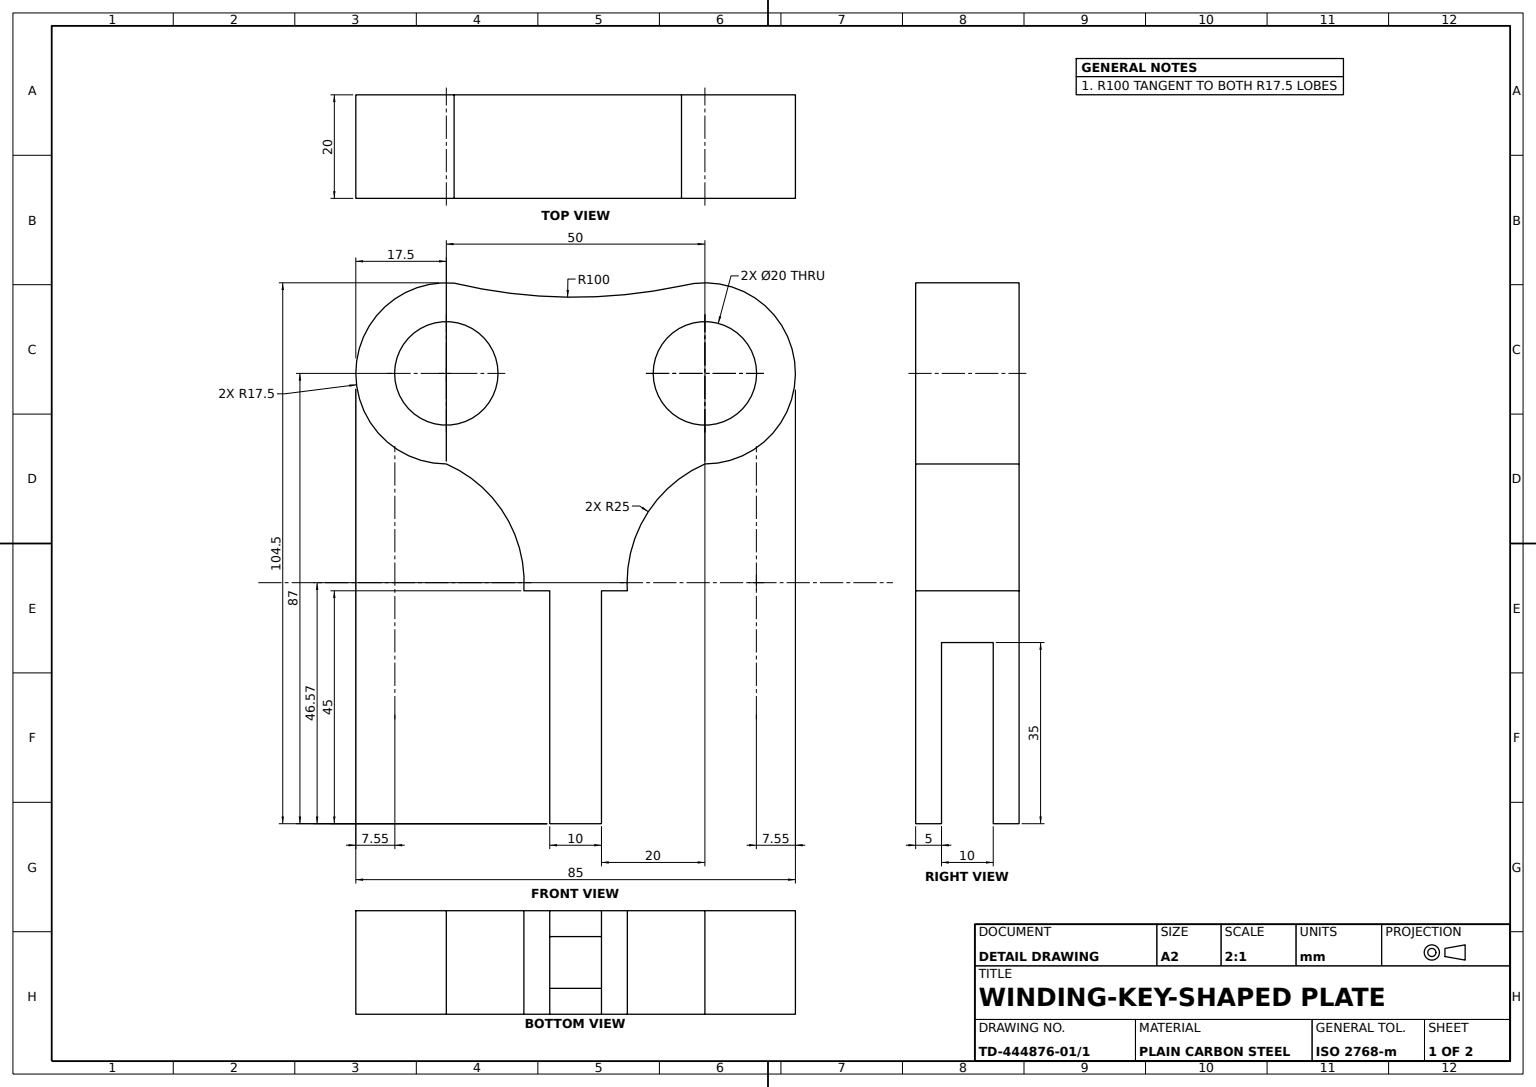
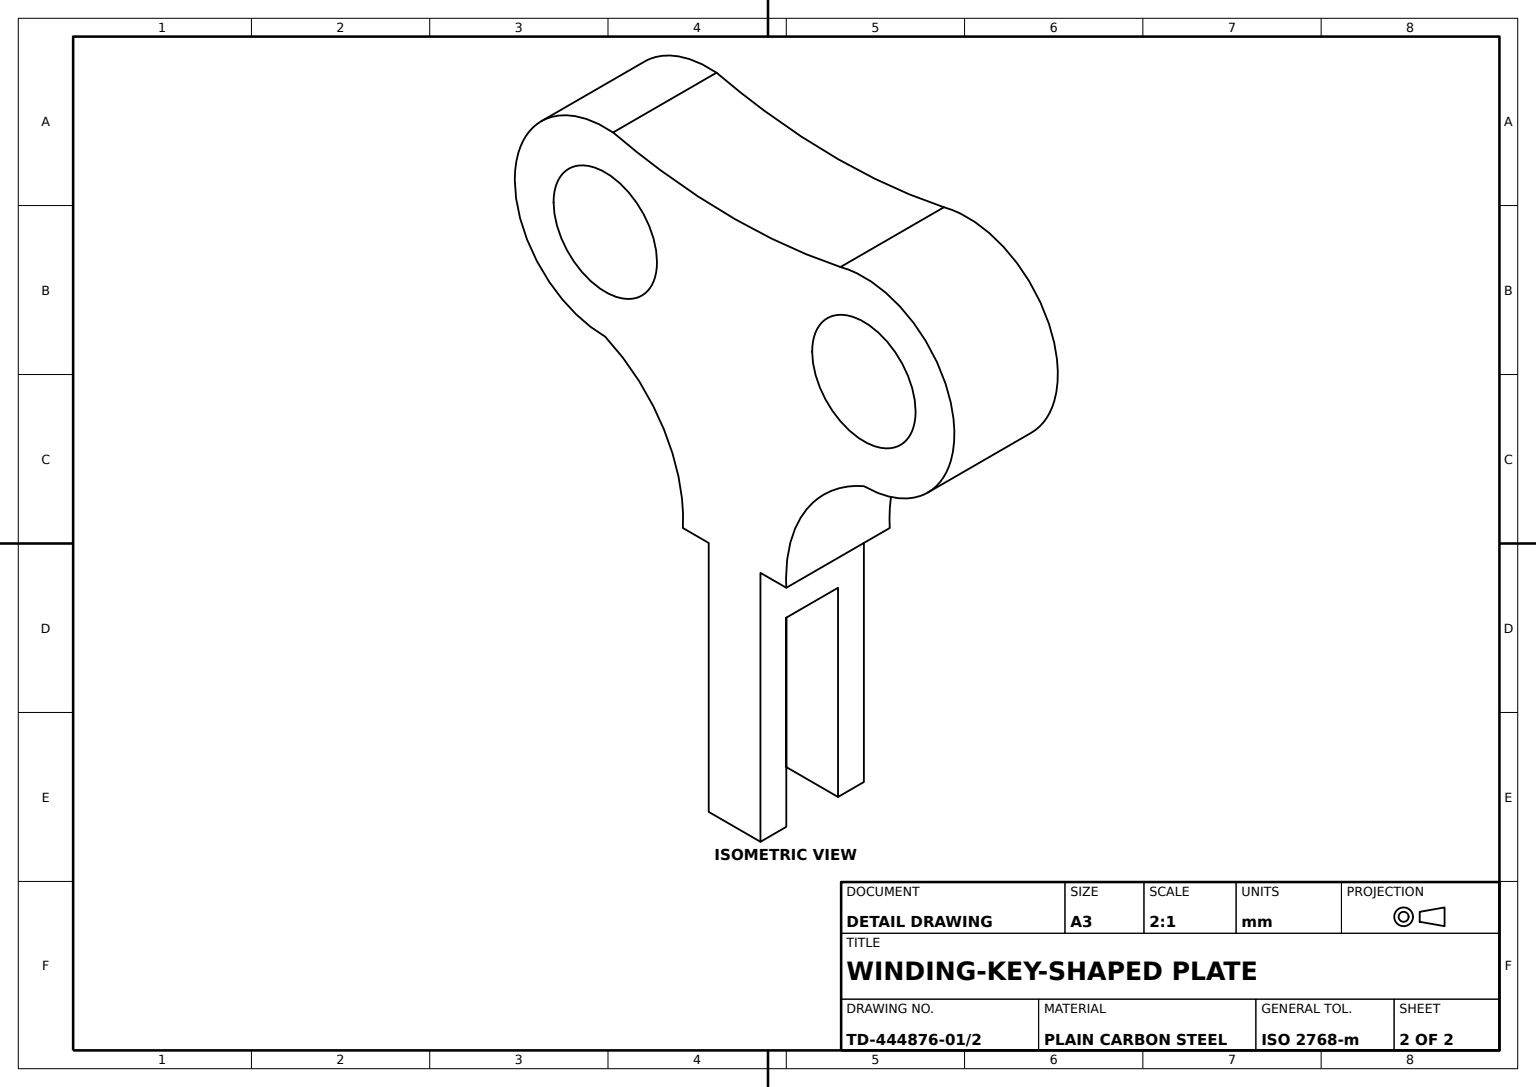
from build123d import *

# Parameters (mm, degrees)
KEY_BODY_DEPTH         = 20
SHANK_SLOT_SKETCH_W    = 10
SHANK_SLOT_SKETCH_H    = 35
SHANK_SLOT_DEPTH       = 20
GRIP_HOLES_SKETCH_R    = 10
GRIP_HOLES_2X_20_DEPTH = 20


with BuildPart() as part:
    # Key Profile Sketch → Key Body (new body)
    with BuildSketch(Plane.XY):
        with BuildLine():
            Line((25, -87), (30, -87))
            Line((30, -87), (30, -42))
            Line((30, -42), (35, -42))
            ThreePointArc((35, -42), (38.629636909, -27.380389945), (50, -17.5))
            ThreePointArc((50, -17.5), (67.350600333, 2.28181246), (45.475335312, 16.904952217))
            ThreePointArc((45.475335312, 16.904952217), (23.461156875, 14.723275331), (1.505978003, 17.435080449))
            ThreePointArc((1.505978003, 17.435080449), (-17.483762579, 0.753688313), (0, -17.5))
            ThreePointArc((0, -17.5), (11.370363091, -27.380389945), (15, -42))
            Line((15, -42), (20, -42))
            Line((20, -42), (20, -87))
            Line((20, -87), (25, -87))
        make_face()
    extrude(amount=KEY_BODY_DEPTH)

    # Shank Slot Sketch → Shank Slot (cut)
    with BuildSketch(Plane(origin=(30, 0, 0), x_dir=(0, 0, -1), z_dir=(1, 0, 0))):
        with Locations((-10, -69.5)):
            Rectangle(SHANK_SLOT_SKETCH_W, SHANK_SLOT_SKETCH_H)
    extrude(amount=-SHANK_SLOT_DEPTH, mode=Mode.SUBTRACT)

    # Grip Holes Sketch → Grip Holes 2xØ20 (cut)
    with BuildSketch(Plane.XY.offset(20)):
        Circle(GRIP_HOLES_SKETCH_R)
        with Locations((50, 0)):
            Circle(GRIP_HOLES_SKETCH_R)
    extrude(amount=-GRIP_HOLES_2X_20_DEPTH, mode=Mode.SUBTRACT)


solid = part.part
